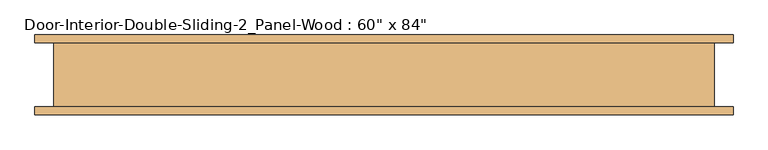
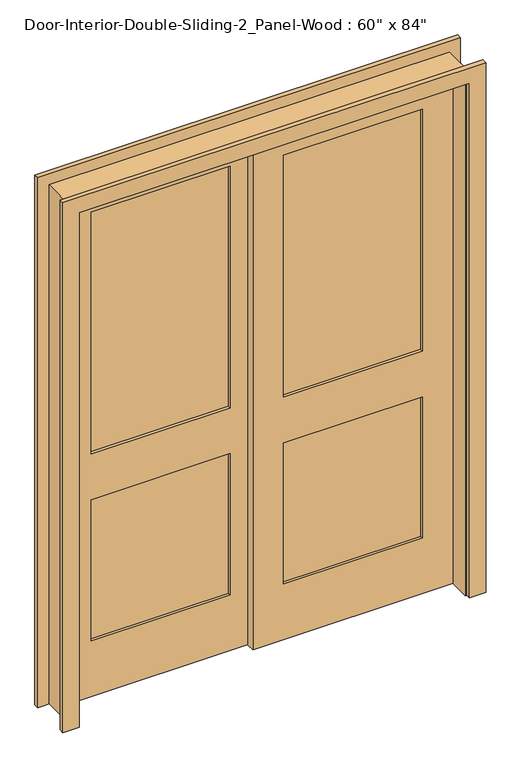
"""IFC4 building model written with IfcOpenShell, lengths in millimetres: door geometry."""

from ifc_helpers import new_model, si_unit, frame, origin, place, context, project, spatial, polyline, outline, extrude, source, transform, mapped, element, save


def door_80d3ddc5(model_context):
    return source(origin(), model_context, "Body", "SweptSolid", [
        extrude(outline(polyline([(641.35, 14.8166667), (95.25, 14.8166667), (95.25, 26.4583333), (641.35, 26.4583333), (641.35, 14.8166667)])), frame((0.0, 0.0, 1009.65), z_axis=(0.0, 0.0, 1.0), x_axis=(1.0, 0.0, 0.0)), (0.0, 0.0, 1.0), 1004.8875),
        extrude(outline(polyline([(641.35, 14.8166667), (95.25, 14.8166667), (95.25, 26.4583333), (641.35, 26.4583333), (641.35, 14.8166667)])), frame((0.0, 0.0, 231.775), z_axis=(0.0, 0.0, 1.0), x_axis=(1.0, 0.0, 0.0)), (0.0, 0.0, 1.0), 587.375),
        extrude(outline(polyline([(2133.6, -25.4), (0.0, -25.4), (0.0, 762.0), (2133.6, 762.0), (2133.6, -25.4)]), holes=[polyline([(2014.5375, 95.25), (2014.5375, 641.35), (1009.65, 641.35), (1009.65, 95.25), (2014.5375, 95.25)]), polyline([(819.15, 95.25), (819.15, 641.35), (231.775, 641.35), (231.775, 95.25), (819.15, 95.25)])]), frame((0.0, 3.175, 0.0), z_axis=(0.0, 1.0, 0.0), x_axis=(0.0, 0.0, 1.0)), (0.0, 0.0, 1.0), 34.925),
        extrude(outline(polyline([(-95.25, 49.7416667), (-641.35, 49.7416667), (-641.35, 61.3833333), (-95.25, 61.3833333), (-95.25, 49.7416667)])), frame((0.0, 0.0, 1009.65), z_axis=(0.0, 0.0, 1.0), x_axis=(1.0, 0.0, 0.0)), (0.0, 0.0, 1.0), 1004.8875),
        extrude(outline(polyline([(-95.25, 49.7416667), (-641.35, 49.7416667), (-641.35, 61.3833333), (-95.25, 61.3833333), (-95.25, 49.7416667)])), frame((0.0, 0.0, 231.775), z_axis=(0.0, 0.0, 1.0), x_axis=(1.0, 0.0, 0.0)), (0.0, 0.0, 1.0), 587.375),
        extrude(outline(polyline([(2133.6, -762.0), (0.0, -762.0), (0.0, 25.4), (2133.6, 25.4), (2133.6, -762.0)]), holes=[polyline([(2014.5375, -641.35), (2014.5375, -95.25), (1009.65, -95.25), (1009.65, -641.35), (2014.5375, -641.35)]), polyline([(819.15, -641.35), (819.15, -95.25), (231.775, -95.25), (231.775, -641.35), (819.15, -641.35)])]), frame((0.0, 38.1, 0.0), z_axis=(0.0, 1.0, 0.0), x_axis=(0.0, 0.0, 1.0)), (0.0, 0.0, 1.0), 34.925),
        extrude(outline(polyline([(0.0, 762.0), (0.0, 787.4), (2159.0, 787.4), (2159.0, -787.4), (0.0, -787.4), (0.0, -762.0), (2133.6, -762.0), (2133.6, 762.0), (0.0, 762.0)])), frame((0.0, -79.375, 0.0), z_axis=(0.0, 1.0, 0.0), x_axis=(0.0, 0.0, 1.0)), (0.0, 0.0, 1.0), 152.4),
        extrude(outline(polyline([(0.0, 768.35), (0.0, 831.85), (2203.45, 831.85), (2203.45, -831.85), (0.0, -831.85), (0.0, -768.35), (2139.95, -768.35), (2139.95, 768.35), (0.0, 768.35)])), frame((0.0, -98.425, 0.0), z_axis=(0.0, 1.0, 0.0), x_axis=(0.0, 0.0, 1.0)), (0.0, 0.0, 1.0), 19.05),
        extrude(outline(polyline([(0.0, 768.35), (0.0, 831.85), (2203.45, 831.85), (2203.45, -831.85), (0.0, -831.85), (0.0, -768.35), (2139.95, -768.35), (2139.95, 768.35), (0.0, 768.35)])), frame((0.0, 73.025, 0.0), z_axis=(0.0, 1.0, 0.0), x_axis=(0.0, 0.0, 1.0)), (0.0, 0.0, 1.0), 19.05),
    ])


if __name__ == "__main__":
    model = new_model("IFC4")
    model_context = context("Model", 3, world=origin())
    ifc_project = project(units=[si_unit("LENGTHUNIT", "METRE", prefix="MILLI")], contexts=[model_context])
    site = spatial("IfcSite", under=ifc_project)
    building = spatial("IfcBuilding", under=site)
    placement = place(None, origin())
    door_shape = door_80d3ddc5(model_context)
    element("IfcDoor", 1, ObjectType="Door-Interior-Double-Sliding-2_Panel-Wood : 60\" x 84\"", at=placement, inside=building, context=model_context, shape_type="MappedRepresentation", body=[
        mapped(door_shape, transform((0.0, 0.0, 0.0), x_axis=(1.0, 0.0, 0.0), y_axis=(0.0, 1.0, 0.0), z_axis=(0.0, 0.0, 1.0))),
    ])
    save(model, "model.ifc")

# Revit data of these elements
# Type "Door-Interior-Double-Sliding-2_Panel-Wood : 60\" x 84\""
#   Type Mark = "8"
#   Assembly Code = "C1020300"
#   Analytic Construction = "Wooden"
#   Top Rail = 0' - 4 11/16"
#   Thickness = 0' - 1 3/8"
#   Thermal Resistance (R) = 2.5876 (h·ft²·°F)/BTU
#   Stiles = 0' - 4 3/4"
#   Rough Width = 5' - 2"
#   Rough Height = 7' - 1"
#   Lock Rail = 0' - 7 1/2"
#   Height = 7' - 0"
#   Width = 5' - 0"
#   Heat Transfer Coefficient (U) = 0.3865 BTU/(h·ft²·°F)
#   Bottom Rail = 0' - 9 1/8"
#   Trim Material = Cherry
#   Panel Material = Cherry
#   Frame Material = Cherry
#   Visual Light Transmittance = 0
#   Solar Heat Gain Coefficient = 0
#   Wall Closure = (empty or 0)
#   Function = (empty or 0)
# Element 1 (IfcDoor, "Door-Interior-Double-Sliding-2_Panel-Wood : 60\" x 84\"")
#   Materials on its faces: "Cherry"
# Materials
#   "Cherry": class "Wood", colour RGB 226 177 128, transparency 0, Description = "Prunus Serotina", Cost = 0
